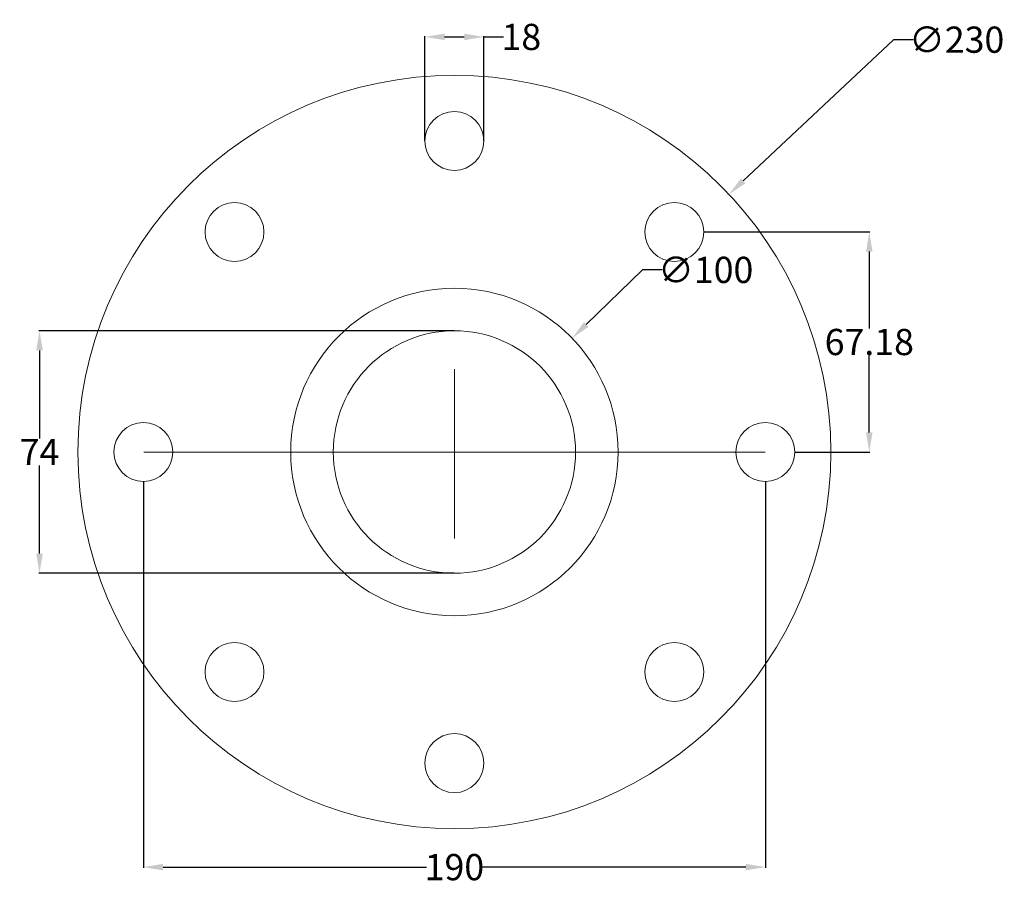
# Model space of a CAD drawing. Units: millimetres. Extents: x 2077 to 2378, y 1360 to 1624.
import ezdxf

# ---------------------------------------------------------------- set-up
doc = ezdxf.new("R2010")
doc.units = ezdxf.units.MM
doc.header["$MEASUREMENT"] = 0
doc.layers.add('M-CONS', color=8, linetype='Continuous', lineweight=13)
doc.layers.add('M-DIMS', color=2, linetype='Continuous', lineweight=18)
doc.styles.get("Standard").update_dxf_attribs({"font": 'arial.ttf'})
doc.dimstyles.get("Standard").update_dxf_attribs({"dimtxt": 8, "dimasz": 6, "dimexe": 0.18, "dimexo": 0.0625, "dimgap": 0.09, "dimtad": 0, "dimtih": 1, "dimtoh": 1, "dimdec": 0, "dimzin": 0, "dimdsep": 46, "dimtxsty": 'Standard', "dimcen": 0.09, "dimadec": 0, "dimazin": 0, "dimtfac": 1, "dimtdec": 0, "dimtofl": 0, "dimtmove": 0, "dimatfit": 3, "dimfxl": 1, "dimtolj": 1, "dimtzin": 0, "dimarcsym": 0})

# ---------------------------------------------------------------- blocks, each defined once
blk = doc.blocks.new('*U1')
blk.add_circle((0, 0), 9)
blk = doc.blocks.new('*U2')
at = {"layer": 'M-CONS', "color": 0, "linetype": 'ByBlock', "lineweight": -2, "transparency": 16777216}
blk.add_blockref('*U1', (2209.97, 1587.16), dxfattribs=at)
for p, rotation in [((2142.79, 1559.34), 45), ((2277.14, 1559.34), 315), ((2114.97, 1492.16), 90), ((2304.97, 1492.16), 270), ((2142.79, 1424.99), 135), ((2277.14, 1424.99), 225), ((2209.97, 1397.16), 180)]:
    blk.add_blockref('*U1', p, dxfattribs=dict(at, rotation=rotation))
blk = doc.blocks.new('*D3')
at = {"layer": 'Defpoints', "color": 0, "transparency": 16777216}
for p in [(2083.216995, 1529.161288), (2209.966995, 1529.161288), (2209.966995, 1455.161288)]:
    blk.add_point(p, dxfattribs=at)
at = {"layer": 'M-DIMS', "color": 0, "lineweight": -2, "transparency": 16777216}
for p, q in [((2209.904495, 1529.161288), (2083.036995, 1529.161288)), ((2083.216995, 1523.161288), (2083.216995, 1496.251288)), ((2083.216995, 1461.161288), (2083.216995, 1488.071288)), ((2209.904495, 1455.161288), (2083.036995, 1455.161288))]:
    blk.add_line(p, q, dxfattribs=at)
at = {"layer": 'M-DIMS', "color": 0, "transparency": 16777216}
for points in [[(2082.216995, 1523.161288), (2084.216995, 1523.161288), (2083.216995, 1529.161288)], [(2082.216995, 1461.161288), (2084.216995, 1461.161288), (2083.216995, 1455.161288)]]:
    blk.add_solid(points, dxfattribs=at)
at = {"layer": 'M-DIMS', "color": 0, "transparency": 16777216, "insert": (2083.216995, 1492.161288), "char_height": 8, "attachment_point": 5}
blk.add_mtext('\\A1;74', dxfattribs=at)
blk = doc.blocks.new('*D4')
at = {"layer": 'Defpoints', "color": 0, "transparency": 16777216}
for p in [(2218.97, 1618.91), (2200.97, 1587.16), (2218.97, 1587.16)]:
    blk.add_point(p, dxfattribs=at)
at = {"layer": 'M-DIMS', "color": 0, "lineweight": -2, "transparency": 16777216}
for p, q in [((2200.97, 1587.22), (2200.97, 1619.09)), ((2206.97, 1618.91), (2212.97, 1618.91)), ((2218.97, 1587.22), (2218.97, 1619.09)), ((2218.97, 1618.91), (2224.97, 1618.91))]:
    blk.add_line(p, q, dxfattribs=at)
at = {"layer": 'M-DIMS', "color": 0, "transparency": 16777216}
for points in [[(2206.97, 1619.91), (2206.97, 1617.91), (2200.97, 1618.91)], [(2212.97, 1619.91), (2212.97, 1617.91), (2218.97, 1618.91)]]:
    blk.add_solid(points, dxfattribs=at)
at = {"layer": 'M-DIMS', "color": 0, "transparency": 16777216, "insert": (2230.42, 1618.91), "char_height": 8, "attachment_point": 5}
blk.add_mtext('\\A1;18', dxfattribs=at)
blk = doc.blocks.new('*D5')
at = {"layer": 'Defpoints', "color": 0, "transparency": 16777216}
for p in [(2114.97, 1483.16), (2304.97, 1483.16), (2304.97, 1365.41)]:
    blk.add_point(p, dxfattribs=at)
at = {"layer": 'M-DIMS', "color": 0, "lineweight": -2, "transparency": 16777216}
for p, q in [((2114.97, 1483.1), (2114.97, 1365.23)), ((2304.97, 1483.1), (2304.97, 1365.23)), ((2120.97, 1365.41), (2201.43, 1365.41)), ((2298.97, 1365.41), (2218.5, 1365.41))]:
    blk.add_line(p, q, dxfattribs=at)
at = {"layer": 'M-DIMS', "color": 0, "transparency": 16777216}
for points in [[(2120.97, 1366.41), (2120.97, 1364.41), (2114.97, 1365.41)], [(2298.97, 1366.41), (2298.97, 1364.41), (2304.97, 1365.41)]]:
    blk.add_solid(points, dxfattribs=at)
at = {"layer": 'M-DIMS', "color": 0, "transparency": 16777216, "insert": (2209.97, 1365.41), "char_height": 8, "attachment_point": 5}
blk.add_mtext('\\A1;190', dxfattribs=at)
blk = doc.blocks.new('*D6')
at = {"layer": 'Defpoints', "color": 0, "transparency": 16777216}
for p in [(2286.14, 1559.34), (2336.72, 1559.34), (2313.97, 1492.16)]:
    blk.add_point(p, dxfattribs=at)
at = {"layer": 'M-DIMS', "color": 0, "lineweight": -2, "transparency": 16777216}
for p, q in [((2286.2, 1559.34), (2336.9, 1559.34)), ((2336.72, 1553.34), (2336.72, 1529.92)), ((2336.72, 1498.16), (2336.72, 1521.57)), ((2314.03, 1492.16), (2336.9, 1492.16))]:
    blk.add_line(p, q, dxfattribs=at)
at = {"layer": 'M-DIMS', "color": 0, "transparency": 16777216}
for points in [[(2335.72, 1553.34), (2337.72, 1553.34), (2336.72, 1559.34)], [(2335.72, 1498.16), (2337.72, 1498.16), (2336.72, 1492.16)]]:
    blk.add_solid(points, dxfattribs=at)
at = {"layer": 'M-DIMS', "color": 0, "transparency": 16777216, "insert": (2336.72, 1525.75), "char_height": 8, "attachment_point": 5}
blk.add_mtext('\\A1;67.18', dxfattribs=at)
blk = doc.blocks.new('*D7')
at = {"layer": 'Defpoints', "color": 0, "transparency": 16777216}
for p in [(2293.83, 1570.85), (2126.1, 1413.48)]:
    blk.add_point(p, dxfattribs=at)
at = {"layer": 'M-DIMS', "color": 0, "lineweight": -2, "transparency": 16777216}
for p, q in [((2344.16, 1618.06), (2298.21, 1574.95)), ((2350.16, 1618.06), (2344.16, 1618.06)), ((2209.88, 1492.16), (2210.06, 1492.16)), ((2209.97, 1492.07), (2209.97, 1492.25))]:
    blk.add_line(p, q, dxfattribs=at)
at = {"layer": 'M-DIMS', "color": 0, "transparency": 16777216}
blk.add_solid([(2297.53, 1575.68), (2298.89, 1574.22), (2293.83, 1570.85)], dxfattribs=at)
at = {"layer": 'M-DIMS', "color": 0, "transparency": 16777216, "insert": (2363.42, 1618.06), "char_height": 8, "attachment_point": 5}
blk.add_mtext('\\A1;∅230', dxfattribs=at)
blk = doc.blocks.new('*D8')
at = {"layer": 'Defpoints', "color": 0, "transparency": 16777216}
for p in [(2245.91, 1526.92), (2174.02, 1457.41)]:
    blk.add_point(p, dxfattribs=at)
at = {"layer": 'M-DIMS', "color": 0, "lineweight": -2, "transparency": 16777216}
for p, q in [((2267.48, 1547.77), (2250.23, 1531.09)), ((2273.48, 1547.77), (2267.48, 1547.77)), ((2209.88, 1492.16), (2210.06, 1492.16)), ((2209.97, 1492.07), (2209.97, 1492.25))]:
    blk.add_line(p, q, dxfattribs=at)
at = {"layer": 'M-DIMS', "color": 0, "transparency": 16777216}
blk.add_solid([(2249.53, 1531.81), (2250.92, 1530.37), (2245.91, 1526.92)], dxfattribs=at)
at = {"layer": 'M-DIMS', "color": 0, "transparency": 16777216, "insert": (2286.75, 1547.77), "char_height": 8, "attachment_point": 5}
blk.add_mtext('\\A1;∅100', dxfattribs=at)

msp = doc.modelspace()

# ---------------------------------------------------------------- linework, layer by layer
at = {"layer": 'M-CONS'}
for p, q in [((2209.967, 1517.464, 61.078), (2209.967, 1465.77, 61.078)), ((2209.967, 1492.161, 61.078), (2169.967, 1492.161, 61.078)), ((2209.967, 1492.161), (2249.967, 1492.161))]:
    msp.add_line(p, q, dxfattribs=at)
at = {"layer": 'M-CONS', "extrusion": (0, -1, 1.8e-15)}
msp.add_line((2209.967, 1492.161, 156), (2209.967, 1492.161, -32), dxfattribs=at)
at = {"layer": 'M-CONS'}
for radius in [115, 50, 50]:
    msp.add_circle((2209.967, 1492.161), radius, dxfattribs=at)
at = {"layer": 'M-CONS', "extrusion": (0, 0, -1)}
for radius in [50, 37]:
    msp.add_circle((-2209.967, 1492.161), radius, dxfattribs=at)
at = {"layer": 'M-CONS', "extrusion": (0, -1, 1.8e-15)}
msp.add_arc((2209.967, 156, -1492.161), 94.922, 180, 0, dxfattribs=at)

# ---------------------------------------------------------------- block references
at = {"layer": 'M-CONS'}
msp.add_blockref('*U2', (0, 0), dxfattribs=at)

# ---------------------------------------------------------------- dimensions: what is measured, and where the dimension line sits
at = {"layer": 'M-DIMS'}
for p1, p2, picture, middle in [((2126.099, 1413.477), (2293.835, 1570.845), '*D7', (2363.422, 1618.056)), ((2174.021, 1457.407), (2245.913, 1526.916), '*D8', (2286.747, 1547.769))]:
    dim = msp.add_diameter_dim_2p(p1=p1, p2=p2, dimstyle='Standard', override={"dimdec": 0, "dimlfac": 1, "dimrnd": 0, "dimzin": 0, "dimdsep": 46, "dimlunit": 2}, dxfattribs=at)
    dim.commit()
    dim.dimension.update_dxf_attribs({"geometry": picture, "text_midpoint": middle, "dimtype": 163})
for base, p1, p2, picture, middle in [((2218.967, 1618.911), (2200.967, 1587.161), (2218.967, 1587.161), '*D4', (2230.419, 1618.911)), ((2304.967, 1365.411), (2114.967, 1483.161), (2304.967, 1483.161), '*D5', (2209.967, 1365.411))]:
    dim = msp.add_linear_dim(base=base, p1=p1, p2=p2, dimstyle='Standard', override={"dimdec": 0, "dimlfac": 1, "dimrnd": 0, "dimzin": 0, "dimdsep": 46, "dimlunit": 2}, dxfattribs=at)
    dim.commit()
    dim.dimension.update_dxf_attribs({"geometry": picture, "text_midpoint": middle})
for base, p1, p2, override, picture, middle in [((2336.717, 1559.3364), (2313.967, 1492.1613), (2286.1421, 1559.3364), {"dimdec": 2, "dimlfac": 1, "dimrnd": 0, "dimzin": 0, "dimdsep": 46, "dimlunit": 2}, '*D6', (2336.717, 1525.7489)), ((2083.217, 1529.161), (2209.967, 1455.161), (2209.967, 1529.161), {"dimdec": 0, "dimlfac": 1, "dimrnd": 0, "dimzin": 0, "dimdsep": 46, "dimlunit": 2}, '*D3', (2083.217, 1492.161))]:
    dim = msp.add_linear_dim(base=base, p1=p1, p2=p2, angle=90, dimstyle='Standard', override=override, dxfattribs=at)
    dim.commit()
    dim.dimension.update_dxf_attribs({"geometry": picture, "text_midpoint": middle})

doc.saveas('drawing.dxf')
